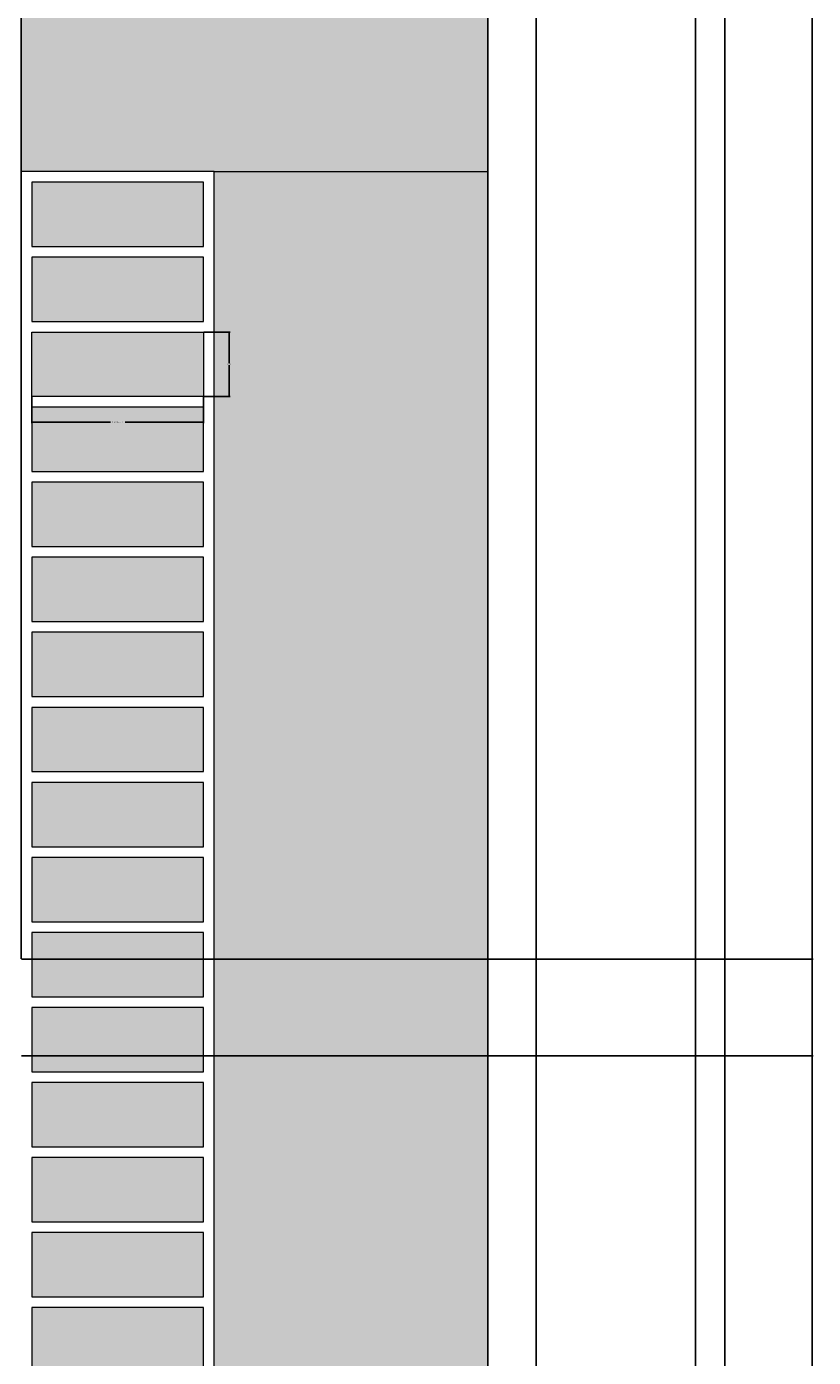
# Model space of a CAD drawing. Units: inches. Extents: x 84 to 1044, y -280 to 906.
# Tile 104 of 105: x 897 to 1044, y 326 to 574. Entities that reach past the tile are written whole.
import ezdxf

# ---------------------------------------------------------------- set-up
doc = ezdxf.new("R2010")
doc.units = ezdxf.units.IN
for name, color, linetype, lineweight in [('A-ANNO-DIMS', 2, 'Continuous', 18), ('A-ANNO-TTLB', 7, 'Continuous', 25), ('C-PROP', 7, 'Continuous', 25), ('L-HRDS', 32, 'Continuous', 18)]:
    doc.layers.add(name, color=color, linetype=linetype, lineweight=lineweight)
doc.layers.add('L-HRDS-PATT', color=23, linetype='Continuous', lineweight=9, true_color=0xc2877b)
doc.layers.add('L-PLNT-PATT', color=9, linetype='Continuous', lineweight=9, true_color=0xafd9aa)
doc.styles.get("Standard").update_dxf_attribs({"font": 'arial.ttf'})
doc.dimstyles.get("Standard").update_dxf_attribs({"dimtxt": 0.18, "dimasz": 0.18, "dimexe": 0.18, "dimexo": 0.0625, "dimgap": 0.09, "dimtad": 0, "dimtih": 1, "dimtoh": 1, "dimdec": 4, "dimzin": 0, "dimdsep": 46, "dimtxsty": 'Standard', "dimcen": 0.09, "dimadec": 0, "dimazin": 0, "dimtfac": 1, "dimtdec": 4, "dimtofl": 0, "dimtmove": 0, "dimatfit": 3, "dimfxl": 1, "dimtolj": 1, "dimtzin": 0, "dimarcsym": 0})

# ---------------------------------------------------------------- blocks, each defined once
blk = doc.blocks.new('PAVER-32X12')
blk.add_lwpolyline([(0, 12), (32, 12), (32, 0), (0, 0)], close=True)
blk = doc.blocks.new('*D32')
at = {"layer": 'A-ANNO-DIMS', "color": 0, "lineweight": -2, "transparency": 16777216}
for p, q in [((898.07, 505.06), (898.07, 500.14)), ((930.07, 505.06), (930.07, 500.14)), ((898.25, 500.32), (912.72, 500.32)), ((929.89, 500.32), (915.43, 500.32))]:
    blk.add_line(p, q, dxfattribs=at)
at = {"layer": 'A-ANNO-DIMS', "color": 0, "transparency": 16777216}
for points in [[(898.25, 500.35), (898.25, 500.29), (898.07, 500.32)], [(929.89, 500.35), (929.89, 500.29), (930.07, 500.32)]]:
    blk.add_solid(points, dxfattribs=at)
at = {"layer": 'Defpoints', "color": 0, "transparency": 16777216}
for p in [(898.07, 505.12), (930.07, 505.12), (930.07, 500.32)]:
    blk.add_point(p, dxfattribs=at)
at = {"layer": 'A-ANNO-DIMS', "color": 0, "transparency": 16777216, "insert": (914.07, 500.32), "char_height": 0.18, "attachment_point": 5}
blk.add_mtext('\\A1;PATH PAVER 32 TYP.', dxfattribs=at)
blk = doc.blocks.new('*D33')
at = {"layer": 'A-ANNO-DIMS', "color": 0, "lineweight": -2, "transparency": 16777216}
for p, q in [((930.14, 517.12), (935.05, 517.12)), ((934.87, 516.94), (934.87, 511.3)), ((934.87, 505.3), (934.87, 510.94)), ((930.14, 505.12), (935.05, 505.12))]:
    blk.add_line(p, q, dxfattribs=at)
at = {"layer": 'A-ANNO-DIMS', "color": 0, "transparency": 16777216}
for points in [[(934.84, 516.94), (934.9, 516.94), (934.87, 517.12)], [(934.84, 505.3), (934.9, 505.3), (934.87, 505.12)]]:
    blk.add_solid(points, dxfattribs=at)
at = {"layer": 'Defpoints', "color": 0, "transparency": 16777216}
for p in [(930.07, 517.12), (934.87, 517.12), (930.07, 505.12)]:
    blk.add_point(p, dxfattribs=at)
at = {"layer": 'A-ANNO-DIMS', "color": 0, "transparency": 16777216, "insert": (934.87, 511.12), "char_height": 0.18, "attachment_point": 5}
blk.add_mtext('\\A1;12 TYP.', dxfattribs=at)
blk = doc.blocks.new('*D63')
at = {"layer": 'A-ANNO-DIMS', "color": 0, "lineweight": -2, "transparency": 16777216}
for p, q in [((833.14, 709.12), (1043.77, 709.12)), ((1043.59, 708.94), (1043.59, 400.3)), ((1043.59, 91.3), (1043.59, 399.94)), ((896.14, 91.12), (1043.77, 91.12))]:
    blk.add_line(p, q, dxfattribs=at)
at = {"layer": 'A-ANNO-DIMS', "color": 0, "transparency": 16777216}
for points in [[(1043.56, 708.94), (1043.62, 708.94), (1043.59, 709.12)], [(1043.56, 91.3), (1043.62, 91.3), (1043.59, 91.12)]]:
    blk.add_solid(points, dxfattribs=at)
at = {"layer": 'Defpoints', "color": 0, "transparency": 16777216}
for p in [(833.07, 709.12), (1043.59, 709.12), (896.07, 91.12)]:
    blk.add_point(p, dxfattribs=at)
at = {"layer": 'A-ANNO-DIMS', "color": 0, "transparency": 16777216, "insert": (1043.59, 400.12), "char_height": 0.18, "attachment_point": 5}
blk.add_mtext('\\A1;618', dxfattribs=at)
blk = doc.blocks.new('*D65')
at = {"layer": 'A-ANNO-DIMS', "color": 0, "lineweight": -2, "transparency": 16777216}
for p, q in [((896.07, 400.18), (896.07, 905.9)), ((896.25, 905.72), (943.86, 905.72)), ((991.89, 905.72), (944.29, 905.72)), ((992.07, 856.18), (992.07, 905.9))]:
    blk.add_line(p, q, dxfattribs=at)
at = {"layer": 'A-ANNO-DIMS', "color": 0, "transparency": 16777216}
for points in [[(896.25, 905.75), (896.25, 905.69), (896.07, 905.72)], [(991.89, 905.75), (991.89, 905.69), (992.07, 905.72)]]:
    blk.add_solid(points, dxfattribs=at)
at = {"layer": 'Defpoints', "color": 0, "transparency": 16777216}
for p in [(896.07, 905.72), (992.07, 856.12), (896.07, 400.12)]:
    blk.add_point(p, dxfattribs=at)
at = {"layer": 'A-ANNO-DIMS', "color": 0, "transparency": 16777216, "insert": (944.07, 905.72), "char_height": 0.18, "attachment_point": 5}
blk.add_mtext('\\A1;96', dxfattribs=at)
blk = doc.blocks.new('*D76')
at = {"layer": 'A-ANNO-DIMS', "color": 0, "lineweight": -2, "transparency": 16777216}
for p, q in [((896.14, 400.12), (1043.77, 400.12)), ((1043.59, 399.94), (1043.59, 391.3)), ((1043.59, 382.3), (1043.59, 390.94)), ((896.14, 382.12), (1043.77, 382.12))]:
    blk.add_line(p, q, dxfattribs=at)
at = {"layer": 'A-ANNO-DIMS', "color": 0, "transparency": 16777216}
for points in [[(1043.56, 399.94), (1043.62, 399.94), (1043.59, 400.12)], [(1043.56, 382.3), (1043.62, 382.3), (1043.59, 382.12)]]:
    blk.add_solid(points, dxfattribs=at)
at = {"layer": 'Defpoints', "color": 0, "transparency": 16777216}
for p in [(896.07, 400.12), (1043.59, 400.12), (896.07, 382.12)]:
    blk.add_point(p, dxfattribs=at)
at = {"layer": 'A-ANNO-DIMS', "color": 0, "transparency": 16777216, "insert": (1043.59, 391.12), "char_height": 0.18, "attachment_point": 5}
blk.add_mtext('\\A1;18', dxfattribs=at)

msp = doc.modelspace()

# ---------------------------------------------------------------- hatches: boundary and pattern name
at = {"layer": 'L-HRDS-PATT', "transparency": 33554597}
h = msp.add_hatch(color=256, dxfattribs=at)
h.dxf.hatch_style = 1
h.paths.add_polyline_path([(930.074, 545.12), (898.074, 545.12), (898.074, 533.12), (930.074, 533.12)])
h.paths.add_polyline_path([(930.074, 531.12), (898.074, 531.12), (898.074, 519.12), (930.074, 519.12)])
h.paths.add_polyline_path([(930.074, 517.12), (898.074, 517.12), (898.074, 505.12), (930.074, 505.12)])
h.paths.add_polyline_path([(930.074, 503.12), (898.074, 503.12), (898.074, 491.12), (930.074, 491.12)])
h.paths.add_polyline_path([(930.074, 489.12), (898.074, 489.12), (898.074, 477.12), (930.074, 477.12)])
h.paths.add_polyline_path([(930.074, 475.12), (898.074, 475.12), (898.074, 463.12), (930.074, 463.12)])
h.paths.add_polyline_path([(930.074, 461.12), (898.074, 461.12), (898.074, 449.12), (930.074, 449.12)])
h.paths.add_polyline_path([(930.074, 447.12), (898.074, 447.12), (898.074, 435.12), (930.074, 435.12)])
h.paths.add_polyline_path([(930.074, 433.12), (898.074, 433.12), (898.074, 421.12), (930.074, 421.12)])
h.paths.add_polyline_path([(930.074, 419.12), (898.074, 419.12), (898.074, 407.12), (930.074, 407.12)])
h.paths.add_polyline_path([(930.074, 405.12), (898.074, 405.12), (898.074, 393.12), (930.074, 393.12)])
h.paths.add_polyline_path([(930.074, 391.12), (898.074, 391.12), (898.074, 379.12), (930.074, 379.12)])
h.paths.add_polyline_path([(930.074, 377.12), (898.074, 377.12), (898.074, 365.12), (930.074, 365.12)])
h.paths.add_polyline_path([(930.074, 363.12), (898.074, 363.12), (898.074, 351.12), (930.074, 351.12)])
h.paths.add_polyline_path([(930.074, 349.12), (898.074, 349.12), (898.074, 337.12), (930.074, 337.12)])
h.paths.add_polyline_path([(930.074, 335.12), (898.074, 335.12), (898.074, 323.12), (930.074, 323.12)])
h.paths.add_polyline_path([(930.074, 321.12), (898.074, 321.12), (898.074, 309.12), (930.074, 309.12)])
h.paths.add_polyline_path([(930.074, 307.12), (898.074, 307.12), (898.074, 295.12), (930.074, 295.12)])
h.paths.add_polyline_path([(930.074, 293.12), (898.074, 293.12), (898.074, 281.12), (930.074, 281.12)])
h.paths.add_polyline_path([(930.074, 279.12), (898.074, 279.12), (898.074, 267.12), (930.074, 267.12)])
at = {"layer": 'L-PLNT-PATT', "transparency": 33554597}
h = msp.add_hatch(color=256, dxfattribs=at)
h.dxf.hatch_style = 1
h.paths.add_polyline_path([(434.074, 769.12), (386.074, 769.12), (386.074, 709.12), (434.074, 709.12)])
h.paths.add_polyline_path([(896.074, 847.12), (434.074, 847.12), (434.074, 769.12), (434.074, 709.12), (470.074, 709.12), (506.074, 709.12), (572.074, 709.12), (608.074, 709.12), (698.074, 709.12), (770.074, 709.12), (833.074, 709.12), (896.074, 709.12)])
h.paths.add_polyline_path([(983.074, 847.12), (896.074, 847.12), (896.074, 709.12), (896.074, 547.12), (932.074, 547.12), (983.074, 547.12)])
h.paths.add_polyline_path([(983.074, 547.12), (932.074, 547.12), (932.074, 265.12), (983.074, 265.12)])
h.paths.add_polyline_path([(203.179, 646.12), (203.179, 709.12), (203.179, 745.12), (143.179, 745.12), (143.179, 271.12), (203.179, 271.12), (203.179, 274.12), (203.179, 310.12), (203.179, 574.12)])

# ---------------------------------------------------------------- linework, layer by layer
at = {"layer": 'A-ANNO-TTLB'}
for points in [[(101.1, 905.916), (1027.308, 905.916), (1027.308, -279.764), (101.1, -279.764)], [(106.576, 900.439), (1021.832, 900.439), (1021.832, -274.288), (106.576, -274.288)]]:
    msp.add_lwpolyline(points, close=True, dxfattribs=at)
at = {"layer": 'C-PROP'}
for points in [[(143.179, -121.88), (134.179, -121.88), (134.179, 856.12), (992.074, 856.12), (992.074, -121.88), (624.574, -121.88)], [(143.179, -112.88), (143.179, 847.12), (983.074, 847.12), (983.074, -112.88), (624.574, -112.88)]]:
    msp.add_lwpolyline(points, dxfattribs=at)
at = {"layer": 'L-HRDS'}
for p, q in [((932.074, 547.12), (896.074, 547.12)), ((932.074, 265.12), (932.074, 547.12)), ((932.074, 547.12), (983.074, 547.12))]:
    msp.add_line(p, q, dxfattribs=at)

# ---------------------------------------------------------------- block references
at = {"layer": 'L-HRDS', "extrusion": (0, 0, -1), "zscale": -1, "rotation": 180}
for p in [(-898.07, 545.12), (-898.07, 531.12), (-898.07, 503.12), (-898.07, 489.12), (-898.07, 475.12), (-898.07, 461.12), (-898.07, 447.12), (-898.07, 433.12), (-898.07, 419.12), (-898.07, 405.12), (-898.07, 391.12), (-898.07, 377.12), (-898.07, 363.12), (-898.07, 349.12), (-898.07, 335.12)]:
    msp.add_blockref('PAVER-32X12', p, dxfattribs=at)
at = {"layer": 'L-HRDS'}
msp.add_blockref('PAVER-32X12', (898.07, 505.12), dxfattribs=at)

# ---------------------------------------------------------------- dimensions: what is measured, and where the dimension line sits
at = {"layer": 'A-ANNO-DIMS'}
dim = msp.add_linear_dim(base=(896.074, 905.72), p1=(992.074, 856.12), p2=(896.074, 400.12), dimstyle='Standard', override={"dimdec": 0, "dimlfac": 1, "dimrnd": 0, "dimzin": 0, "dimdsep": 46, "dimlunit": 2}, dxfattribs=at)
dim.commit()
dim.dimension.update_dxf_attribs({"geometry": '*D65', "text_midpoint": (944.074, 905.72)})
for base, p1, p2, picture, middle in [((1043.588, 709.12), (896.074, 91.12), (833.074, 709.12), '*D63', (1043.588, 400.12)), ((1043.588, 400.12), (896.074, 382.12), (896.074, 400.12), '*D76', (1043.588, 391.12))]:
    dim = msp.add_linear_dim(base=base, p1=p1, p2=p2, angle=90, dimstyle='Standard', override={"dimdec": 0, "dimlfac": 1, "dimrnd": 0, "dimzin": 0, "dimdsep": 46, "dimlunit": 2}, dxfattribs=at)
    dim.commit()
    dim.dimension.update_dxf_attribs({"geometry": picture, "text_midpoint": middle})
dim = msp.add_linear_dim(base=(934.874, 517.12), p1=(930.074, 505.12), p2=(930.074, 517.12), angle=90, text='<> TYP.', dimstyle='Standard', override={"dimdec": 0, "dimlfac": 1, "dimrnd": 0, "dimzin": 0, "dimdsep": 46, "dimlunit": 2}, dxfattribs=at)
dim.commit()
dim.dimension.update_dxf_attribs({"geometry": '*D33', "text_midpoint": (934.874, 511.12)})
dim = msp.add_linear_dim(base=(930.074, 500.32), p1=(898.074, 505.12), p2=(930.074, 505.12), text='PATH PAVER <> TYP.', dimstyle='Standard', override={"dimdec": 0, "dimlfac": 1, "dimrnd": 0, "dimzin": 0, "dimdsep": 46, "dimlunit": 2}, dxfattribs=at)
dim.commit()
dim.dimension.update_dxf_attribs({"geometry": '*D32', "text_midpoint": (914.074, 500.32)})

doc.saveas('drawing.dxf')
